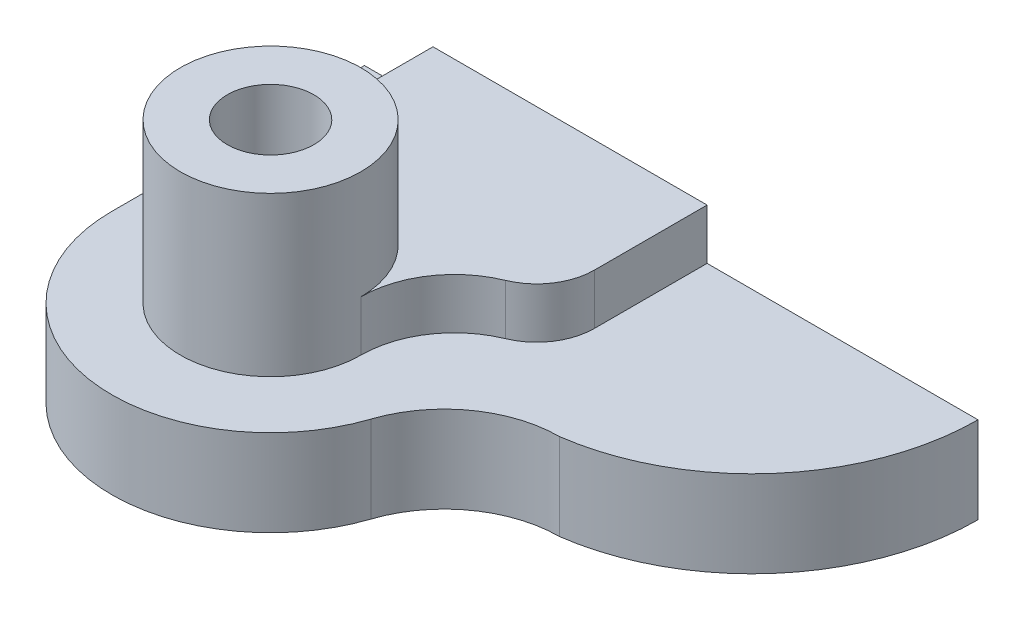
ISO-10303-21;
HEADER;
FILE_DESCRIPTION(('STEP AP214'),'2;1');
FILE_NAME('part.step','',(''),(''),'','','');
FILE_SCHEMA(('AUTOMOTIVE_DESIGN { 1 0 10303 214 1 1 1 1 }'));
ENDSEC;
DATA;
#1=APPLICATION_CONTEXT('core data for automotive mechanical design processes');
#2=APPLICATION_PROTOCOL_DEFINITION('international standard','automotive_design',2000,#1);
#3=PRODUCT_CONTEXT('',#1,'mechanical');
#4=PRODUCT('Part','Part','',(#3));
#5=PRODUCT_RELATED_PRODUCT_CATEGORY('part','',(#4));
#6=PRODUCT_DEFINITION_FORMATION('','',#4);
#7=PRODUCT_DEFINITION_CONTEXT('part definition',#1,'design');
#8=PRODUCT_DEFINITION('design','',#6,#7);
#9=PRODUCT_DEFINITION_SHAPE('','',#8);
#10=(LENGTH_UNIT() NAMED_UNIT(*) SI_UNIT(.MILLI.,.METRE.));
#11=(NAMED_UNIT(*) PLANE_ANGLE_UNIT() SI_UNIT($,.RADIAN.));
#12=(NAMED_UNIT(*) SI_UNIT($,.STERADIAN.) SOLID_ANGLE_UNIT());
#13=UNCERTAINTY_MEASURE_WITH_UNIT(LENGTH_MEASURE(1.E-05),#10,'distance_accuracy_value','');
#14=(GEOMETRIC_REPRESENTATION_CONTEXT(3) GLOBAL_UNCERTAINTY_ASSIGNED_CONTEXT((#13)) GLOBAL_UNIT_ASSIGNED_CONTEXT((#10,
#11,#12)) REPRESENTATION_CONTEXT('',''));
#15=CARTESIAN_POINT('',(0.,0.,0.));
#16=DIRECTION('',(0.,0.,1.));
#17=DIRECTION('',(1.,0.,0.));
#18=AXIS2_PLACEMENT_3D('',#15,#16,#17);
#19=CARTESIAN_POINT('',(36.0555127546399,12.,12.));
#20=DIRECTION('',(0.,-1.,0.));
#21=DIRECTION('',(0.,0.,-1.));
#22=AXIS2_PLACEMENT_3D('',#19,#20,#21);
#23=CYLINDRICAL_SURFACE('',#22,16.);
#24=CARTESIAN_POINT('',(36.0555127546399,0.,12.));
#25=DIRECTION('',(0.,1.,0.));
#26=DIRECTION('',(0.,0.,1.));
#27=AXIS2_PLACEMENT_3D('',#24,#25,#26);
#28=CIRCLE('',#27,16.);
#29=CARTESIAN_POINT('',(36.0555127546399,0.,-4.));
#30=VERTEX_POINT('',#29);
#31=CARTESIAN_POINT('',(20.8742442263705,0.,6.94736842105262));
#32=VERTEX_POINT('',#31);
#33=EDGE_CURVE('E132',#30,#32,#28,.T.);
#34=ORIENTED_EDGE('',*,*,#33,.F.);
#35=DIRECTION('',(0.,-1.,0.));
#36=VECTOR('',#35,1.);
#37=CARTESIAN_POINT('',(36.0555127546399,12.,-4.));
#38=LINE('',#37,#36);
#39=CARTESIAN_POINT('',(36.0555127546399,12.,-4.));
#40=VERTEX_POINT('',#39);
#41=EDGE_CURVE('E11',#40,#30,#38,.T.);
#42=ORIENTED_EDGE('',*,*,#41,.F.);
#43=CARTESIAN_POINT('',(36.0555127546399,12.,12.));
#44=DIRECTION('',(0.,1.,0.));
#45=DIRECTION('',(0.,0.,1.));
#46=AXIS2_PLACEMENT_3D('',#43,#44,#45);
#47=CIRCLE('',#46,16.);
#48=CARTESIAN_POINT('',(20.8742442263705,12.,6.94736842105262));
#49=VERTEX_POINT('',#48);
#50=EDGE_CURVE('E141',#40,#49,#47,.T.);
#51=ORIENTED_EDGE('',*,*,#50,.T.);
#52=DIRECTION('',(0.,-1.,0.));
#53=VECTOR('',#52,1.);
#54=CARTESIAN_POINT('',(20.8742442263705,12.,6.94736842105262));
#55=LINE('',#54,#53);
#56=EDGE_CURVE('E81',#49,#32,#55,.T.);
#57=ORIENTED_EDGE('',*,*,#56,.T.);
#58=EDGE_LOOP('',(#34,#42,#51,#57));
#59=FACE_BOUND('',#58,.T.);
#60=ADVANCED_FACE('F41',(#59),#23,.F.);
#61=CARTESIAN_POINT('',(31.6947950140361,12.,-35.));
#62=DIRECTION('',(0.,-1.,0.));
#63=DIRECTION('',(0.,0.,-1.));
#64=AXIS2_PLACEMENT_3D('',#61,#62,#63);
#65=CYLINDRICAL_SURFACE('',#64,31.3052049859639);
#66=CARTESIAN_POINT('',(31.6947950140361,0.,-35.));
#67=DIRECTION('',(0.,1.,0.));
#68=DIRECTION('',(0.,0.,1.));
#69=AXIS2_PLACEMENT_3D('',#66,#67,#68);
#70=CIRCLE('',#69,31.3052049859639);
#71=CARTESIAN_POINT('',(63.,0.,-35.));
#72=VERTEX_POINT('',#71);
#73=EDGE_CURVE('E135',#72,#30,#70,.F.);
#74=ORIENTED_EDGE('',*,*,#73,.F.);
#75=DIRECTION('',(0.,-1.,0.));
#76=VECTOR('',#75,1.);
#77=CARTESIAN_POINT('',(63.,12.,-35.));
#78=LINE('',#77,#76);
#79=CARTESIAN_POINT('',(63.,12.,-35.));
#80=VERTEX_POINT('',#79);
#81=EDGE_CURVE('E47',#80,#72,#78,.T.);
#82=ORIENTED_EDGE('',*,*,#81,.F.);
#83=CARTESIAN_POINT('',(31.6947950140361,12.,-35.));
#84=DIRECTION('',(0.,1.,0.));
#85=DIRECTION('',(0.,0.,1.));
#86=AXIS2_PLACEMENT_3D('',#83,#84,#85);
#87=CIRCLE('',#86,31.3052049859639);
#88=EDGE_CURVE('E159',#80,#40,#87,.F.);
#89=ORIENTED_EDGE('',*,*,#88,.T.);
#90=ORIENTED_EDGE('',*,*,#41,.T.);
#91=EDGE_LOOP('',(#74,#82,#89,#90));
#92=FACE_BOUND('',#91,.T.);
#93=ADVANCED_FACE('F153',(#92),#65,.T.);
#94=CARTESIAN_POINT('',(0.,12.,-35.));
#95=DIRECTION('',(0.,0.,-1.));
#96=DIRECTION('',(-1.,0.,0.));
#97=AXIS2_PLACEMENT_3D('',#94,#95,#96);
#98=PLANE('',#97);
#99=DIRECTION('',(1.,0.,0.));
#100=VECTOR('',#99,1.);
#101=CARTESIAN_POINT('',(0.,0.,-35.));
#102=LINE('',#101,#100);
#103=CARTESIAN_POINT('',(-22.,0.,-35.));
#104=VERTEX_POINT('',#103);
#105=EDGE_CURVE('E113',#104,#72,#102,.T.);
#106=ORIENTED_EDGE('',*,*,#105,.F.);
#107=DIRECTION('',(0.,-1.,0.));
#108=VECTOR('',#107,1.);
#109=CARTESIAN_POINT('',(-22.,12.,-35.));
#110=LINE('',#109,#108);
#111=CARTESIAN_POINT('',(-22.,12.,-35.));
#112=VERTEX_POINT('',#111);
#113=EDGE_CURVE('E107',#112,#104,#110,.T.);
#114=ORIENTED_EDGE('',*,*,#113,.F.);
#115=DIRECTION('',(1.,0.,0.));
#116=VECTOR('',#115,1.);
#117=CARTESIAN_POINT('',(0.,12.,-35.));
#118=LINE('',#117,#116);
#119=CARTESIAN_POINT('',(-12.5,12.,-35.));
#120=VERTEX_POINT('',#119);
#121=EDGE_CURVE('E114',#112,#120,#118,.T.);
#122=ORIENTED_EDGE('',*,*,#121,.T.);
#123=DIRECTION('',(0.,-1.,0.));
#124=VECTOR('',#123,1.);
#125=CARTESIAN_POINT('',(-12.5,19.,-35.));
#126=LINE('',#125,#124);
#127=CARTESIAN_POINT('',(-12.5,19.,-35.));
#128=VERTEX_POINT('',#127);
#129=EDGE_CURVE('E220',#128,#120,#126,.T.);
#130=ORIENTED_EDGE('',*,*,#129,.F.);
#131=DIRECTION('',(1.,0.,0.));
#132=VECTOR('',#131,1.);
#133=CARTESIAN_POINT('',(0.,19.,-35.));
#134=LINE('',#133,#132);
#135=CARTESIAN_POINT('',(25.4725075103815,19.,-35.));
#136=VERTEX_POINT('',#135);
#137=EDGE_CURVE('E212',#128,#136,#134,.T.);
#138=ORIENTED_EDGE('',*,*,#137,.T.);
#139=DIRECTION('',(0.,-1.,0.));
#140=VECTOR('',#139,1.);
#141=CARTESIAN_POINT('',(25.4725075103815,19.,-35.));
#142=LINE('',#141,#140);
#143=CARTESIAN_POINT('',(25.4725075103815,12.,-35.));
#144=VERTEX_POINT('',#143);
#145=EDGE_CURVE('E221',#136,#144,#142,.T.);
#146=ORIENTED_EDGE('',*,*,#145,.T.);
#147=DIRECTION('',(1.,0.,0.));
#148=VECTOR('',#147,1.);
#149=CARTESIAN_POINT('',(0.,12.,-35.));
#150=LINE('',#149,#148);
#151=EDGE_CURVE('E149',#144,#80,#150,.T.);
#152=ORIENTED_EDGE('',*,*,#151,.T.);
#153=ORIENTED_EDGE('',*,*,#81,.T.);
#154=EDGE_LOOP('',(#106,#114,#122,#130,#138,#146,#152,#153));
#155=FACE_BOUND('',#154,.T.);
#156=ADVANCED_FACE('F109',(#155),#98,.T.);
#157=CARTESIAN_POINT('',(-22.,12.,0.));
#158=DIRECTION('',(1.,0.,0.));
#159=DIRECTION('',(0.,0.,-1.));
#160=AXIS2_PLACEMENT_3D('',#157,#158,#159);
#161=PLANE('',#160);
#162=DIRECTION('',(0.,0.,1.));
#163=VECTOR('',#162,1.);
#164=CARTESIAN_POINT('',(-22.,0.,0.));
#165=LINE('',#164,#163);
#166=CARTESIAN_POINT('',(-22.,0.,0.));
#167=VERTEX_POINT('',#166);
#168=EDGE_CURVE('E76',#104,#167,#165,.T.);
#169=ORIENTED_EDGE('',*,*,#168,.T.);
#170=DIRECTION('',(0.,-1.,0.));
#171=VECTOR('',#170,1.);
#172=CARTESIAN_POINT('',(-22.,12.,0.));
#173=LINE('',#172,#171);
#174=CARTESIAN_POINT('',(-22.,12.,0.));
#175=VERTEX_POINT('',#174);
#176=EDGE_CURVE('E116',#175,#167,#173,.T.);
#177=ORIENTED_EDGE('',*,*,#176,.F.);
#178=DIRECTION('',(0.,0.,1.));
#179=VECTOR('',#178,1.);
#180=CARTESIAN_POINT('',(-22.,12.,0.));
#181=LINE('',#180,#179);
#182=EDGE_CURVE('E119',#112,#175,#181,.T.);
#183=ORIENTED_EDGE('',*,*,#182,.F.);
#184=ORIENTED_EDGE('',*,*,#113,.T.);
#185=EDGE_LOOP('',(#169,#177,#183,#184));
#186=FACE_BOUND('',#185,.T.);
#187=ADVANCED_FACE('F118',(#186),#161,.F.);
#188=CARTESIAN_POINT('',(0.,12.,0.));
#189=DIRECTION('',(0.,-1.,0.));
#190=DIRECTION('',(0.,0.,-1.));
#191=AXIS2_PLACEMENT_3D('',#188,#189,#190);
#192=CYLINDRICAL_SURFACE('',#191,22.);
#193=CARTESIAN_POINT('',(0.,0.,0.));
#194=DIRECTION('',(0.,1.,0.));
#195=DIRECTION('',(0.,0.,1.));
#196=AXIS2_PLACEMENT_3D('',#193,#194,#195);
#197=CIRCLE('',#196,22.);
#198=EDGE_CURVE('E143',#167,#32,#197,.T.);
#199=ORIENTED_EDGE('',*,*,#198,.T.);
#200=ORIENTED_EDGE('',*,*,#56,.F.);
#201=CARTESIAN_POINT('',(0.,12.,0.));
#202=DIRECTION('',(0.,1.,0.));
#203=DIRECTION('',(0.,0.,1.));
#204=AXIS2_PLACEMENT_3D('',#201,#202,#203);
#205=CIRCLE('',#204,22.);
#206=EDGE_CURVE('E60',#175,#49,#205,.T.);
#207=ORIENTED_EDGE('',*,*,#206,.F.);
#208=ORIENTED_EDGE('',*,*,#176,.T.);
#209=EDGE_LOOP('',(#199,#200,#207,#208));
#210=FACE_BOUND('',#209,.T.);
#211=ADVANCED_FACE('F157',(#210),#192,.T.);
#212=CARTESIAN_POINT('',(0.,12.,0.));
#213=DIRECTION('',(0.,1.,0.));
#214=DIRECTION('',(0.,0.,1.));
#215=AXIS2_PLACEMENT_3D('',#212,#213,#214);
#216=PLANE('',#215);
#217=ORIENTED_EDGE('',*,*,#50,.F.);
#218=ORIENTED_EDGE('',*,*,#88,.F.);
#219=ORIENTED_EDGE('',*,*,#151,.F.);
#220=DIRECTION('',(0.,0.,-1.));
#221=VECTOR('',#220,1.);
#222=CARTESIAN_POINT('',(25.4725075103815,12.,0.));
#223=LINE('',#222,#221);
#224=CARTESIAN_POINT('',(25.4725075103815,12.,-19.3867498893706));
#225=VERTEX_POINT('',#224);
#226=EDGE_CURVE('E170',#225,#144,#223,.T.);
#227=ORIENTED_EDGE('',*,*,#226,.F.);
#228=CARTESIAN_POINT('',(17.4725075103815,12.,-19.3867498893706));
#229=DIRECTION('',(0.,1.,0.));
#230=DIRECTION('',(0.,0.,1.));
#231=AXIS2_PLACEMENT_3D('',#228,#229,#230);
#232=CIRCLE('',#231,8.);
#233=CARTESIAN_POINT('',(20.5241216279743,12.,-11.9916399322902));
#234=VERTEX_POINT('',#233);
#235=EDGE_CURVE('E168',#234,#225,#232,.T.);
#236=ORIENTED_EDGE('',*,*,#235,.F.);
#237=CARTESIAN_POINT('',(25.4725075103815,12.,0.));
#238=DIRECTION('',(0.,1.,0.));
#239=DIRECTION('',(0.,0.,1.));
#240=AXIS2_PLACEMENT_3D('',#237,#238,#239);
#241=CIRCLE('',#240,12.9725075103815);
#242=CARTESIAN_POINT('',(12.5,12.,0.));
#243=VERTEX_POINT('',#242);
#244=EDGE_CURVE('E174',#234,#243,#241,.T.);
#245=ORIENTED_EDGE('',*,*,#244,.T.);
#246=CARTESIAN_POINT('',(0.,12.,0.));
#247=DIRECTION('',(0.,1.,0.));
#248=DIRECTION('',(0.,0.,1.));
#249=AXIS2_PLACEMENT_3D('',#246,#247,#248);
#250=CIRCLE('',#249,12.5);
#251=CARTESIAN_POINT('',(-12.5,12.,0.));
#252=VERTEX_POINT('',#251);
#253=EDGE_CURVE('E130',#252,#243,#250,.T.);
#254=ORIENTED_EDGE('',*,*,#253,.F.);
#255=DIRECTION('',(0.,0.,-1.));
#256=VECTOR('',#255,1.);
#257=CARTESIAN_POINT('',(-12.5,12.,0.));
#258=LINE('',#257,#256);
#259=EDGE_CURVE('E124',#252,#120,#258,.T.);
#260=ORIENTED_EDGE('',*,*,#259,.T.);
#261=ORIENTED_EDGE('',*,*,#121,.F.);
#262=ORIENTED_EDGE('',*,*,#182,.T.);
#263=ORIENTED_EDGE('',*,*,#206,.T.);
#264=EDGE_LOOP('',(#217,#218,#219,#227,#236,#245,#254,#260,#261,#262,#263));
#265=FACE_BOUND('',#264,.T.);
#266=ADVANCED_FACE('F125',(#265),#216,.T.);
#267=CARTESIAN_POINT('',(0.,0.,0.));
#268=DIRECTION('',(0.,1.,0.));
#269=DIRECTION('',(0.,0.,1.));
#270=AXIS2_PLACEMENT_3D('',#267,#268,#269);
#271=PLANE('',#270);
#272=ORIENTED_EDGE('',*,*,#105,.T.);
#273=ORIENTED_EDGE('',*,*,#73,.T.);
#274=ORIENTED_EDGE('',*,*,#33,.T.);
#275=ORIENTED_EDGE('',*,*,#198,.F.);
#276=ORIENTED_EDGE('',*,*,#168,.F.);
#277=EDGE_LOOP('',(#272,#273,#274,#275,#276));
#278=FACE_BOUND('',#277,.T.);
#279=CARTESIAN_POINT('',(0.,0.,0.));
#280=DIRECTION('',(0.,1.,0.));
#281=DIRECTION('',(0.,0.,1.));
#282=AXIS2_PLACEMENT_3D('',#279,#280,#281);
#283=CIRCLE('',#282,6.);
#284=CARTESIAN_POINT('',(0.,0.,6.));
#285=VERTEX_POINT('',#284);
#286=EDGE_CURVE('E415',#285,#285,#283,.T.);
#287=ORIENTED_EDGE('',*,*,#286,.T.);
#288=EDGE_LOOP('',(#287));
#289=FACE_BOUND('',#288,.T.);
#290=ADVANCED_FACE('F154',(#278,#289),#271,.F.);
#291=CARTESIAN_POINT('',(25.4725075103815,19.,0.));
#292=DIRECTION('',(0.,-1.,0.));
#293=DIRECTION('',(0.,0.,-1.));
#294=AXIS2_PLACEMENT_3D('',#291,#292,#293);
#295=CYLINDRICAL_SURFACE('',#294,12.9725075103815);
#296=DIRECTION('',(0.,-1.,0.));
#297=VECTOR('',#296,1.);
#298=CARTESIAN_POINT('',(12.5,19.,0.));
#299=LINE('',#298,#297);
#300=CARTESIAN_POINT('',(12.5,19.,0.));
#301=VERTEX_POINT('',#300);
#302=EDGE_CURVE('E181',#301,#243,#299,.T.);
#303=ORIENTED_EDGE('',*,*,#302,.T.);
#304=ORIENTED_EDGE('',*,*,#244,.F.);
#305=DIRECTION('',(0.,-1.,0.));
#306=VECTOR('',#305,1.);
#307=CARTESIAN_POINT('',(20.5241216279743,19.,-11.9916399322902));
#308=LINE('',#307,#306);
#309=CARTESIAN_POINT('',(20.5241216279743,19.,-11.9916399322902));
#310=VERTEX_POINT('',#309);
#311=EDGE_CURVE('E138',#310,#234,#308,.T.);
#312=ORIENTED_EDGE('',*,*,#311,.F.);
#313=CARTESIAN_POINT('',(25.4725075103815,19.,0.));
#314=DIRECTION('',(0.,1.,0.));
#315=DIRECTION('',(0.,0.,1.));
#316=AXIS2_PLACEMENT_3D('',#313,#314,#315);
#317=CIRCLE('',#316,12.9725075103815);
#318=EDGE_CURVE('E240',#310,#301,#317,.T.);
#319=ORIENTED_EDGE('',*,*,#318,.T.);
#320=EDGE_LOOP('',(#303,#304,#312,#319));
#321=FACE_BOUND('',#320,.T.);
#322=ADVANCED_FACE('F237',(#321),#295,.F.);
#323=CARTESIAN_POINT('',(17.4725075103815,19.,-19.3867498893706));
#324=DIRECTION('',(0.,-1.,0.));
#325=DIRECTION('',(0.,0.,-1.));
#326=AXIS2_PLACEMENT_3D('',#323,#324,#325);
#327=CYLINDRICAL_SURFACE('',#326,8.);
#328=ORIENTED_EDGE('',*,*,#235,.T.);
#329=DIRECTION('',(0.,-1.,0.));
#330=VECTOR('',#329,1.);
#331=CARTESIAN_POINT('',(25.4725075103815,19.,-19.3867498893706));
#332=LINE('',#331,#330);
#333=CARTESIAN_POINT('',(25.4725075103815,19.,-19.3867498893706));
#334=VERTEX_POINT('',#333);
#335=EDGE_CURVE('E223',#334,#225,#332,.T.);
#336=ORIENTED_EDGE('',*,*,#335,.F.);
#337=CARTESIAN_POINT('',(17.4725075103815,19.,-19.3867498893706));
#338=DIRECTION('',(0.,1.,0.));
#339=DIRECTION('',(0.,0.,1.));
#340=AXIS2_PLACEMENT_3D('',#337,#338,#339);
#341=CIRCLE('',#340,8.);
#342=EDGE_CURVE('E232',#310,#334,#341,.T.);
#343=ORIENTED_EDGE('',*,*,#342,.F.);
#344=ORIENTED_EDGE('',*,*,#311,.T.);
#345=EDGE_LOOP('',(#328,#336,#343,#344));
#346=FACE_BOUND('',#345,.T.);
#347=ADVANCED_FACE('F231',(#346),#327,.T.);
#348=CARTESIAN_POINT('',(25.4725075103815,19.,0.));
#349=DIRECTION('',(-1.,0.,0.));
#350=DIRECTION('',(0.,0.,1.));
#351=AXIS2_PLACEMENT_3D('',#348,#349,#350);
#352=PLANE('',#351);
#353=ORIENTED_EDGE('',*,*,#226,.T.);
#354=ORIENTED_EDGE('',*,*,#145,.F.);
#355=DIRECTION('',(0.,0.,-1.));
#356=VECTOR('',#355,1.);
#357=CARTESIAN_POINT('',(25.4725075103815,19.,0.));
#358=LINE('',#357,#356);
#359=EDGE_CURVE('E238',#334,#136,#358,.T.);
#360=ORIENTED_EDGE('',*,*,#359,.F.);
#361=ORIENTED_EDGE('',*,*,#335,.T.);
#362=EDGE_LOOP('',(#353,#354,#360,#361));
#363=FACE_BOUND('',#362,.T.);
#364=ADVANCED_FACE('F246',(#363),#352,.F.);
#365=CARTESIAN_POINT('',(-12.5,19.,0.));
#366=DIRECTION('',(-1.,0.,0.));
#367=DIRECTION('',(0.,0.,1.));
#368=AXIS2_PLACEMENT_3D('',#365,#366,#367);
#369=PLANE('',#368);
#370=ORIENTED_EDGE('',*,*,#129,.T.);
#371=ORIENTED_EDGE('',*,*,#259,.F.);
#372=DIRECTION('',(0.,-1.,0.));
#373=VECTOR('',#372,1.);
#374=CARTESIAN_POINT('',(-12.5,19.,0.));
#375=LINE('',#374,#373);
#376=CARTESIAN_POINT('',(-12.5,19.,0.));
#377=VERTEX_POINT('',#376);
#378=EDGE_CURVE('E186',#377,#252,#375,.T.);
#379=ORIENTED_EDGE('',*,*,#378,.F.);
#380=DIRECTION('',(0.,0.,-1.));
#381=VECTOR('',#380,1.);
#382=CARTESIAN_POINT('',(-12.5,19.,0.));
#383=LINE('',#382,#381);
#384=EDGE_CURVE('E207',#377,#128,#383,.T.);
#385=ORIENTED_EDGE('',*,*,#384,.T.);
#386=EDGE_LOOP('',(#370,#371,#379,#385));
#387=FACE_BOUND('',#386,.T.);
#388=ADVANCED_FACE('F216',(#387),#369,.T.);
#389=CARTESIAN_POINT('',(0.,19.,0.));
#390=DIRECTION('',(0.,1.,0.));
#391=DIRECTION('',(0.,0.,1.));
#392=AXIS2_PLACEMENT_3D('',#389,#390,#391);
#393=PLANE('',#392);
#394=ORIENTED_EDGE('',*,*,#318,.F.);
#395=ORIENTED_EDGE('',*,*,#342,.T.);
#396=ORIENTED_EDGE('',*,*,#359,.T.);
#397=ORIENTED_EDGE('',*,*,#137,.F.);
#398=ORIENTED_EDGE('',*,*,#384,.F.);
#399=CARTESIAN_POINT('',(0.,19.,0.));
#400=DIRECTION('',(0.,1.,0.));
#401=DIRECTION('',(0.,0.,1.));
#402=AXIS2_PLACEMENT_3D('',#399,#400,#401);
#403=CIRCLE('',#402,12.5);
#404=EDGE_CURVE('E215',#301,#377,#403,.T.);
#405=ORIENTED_EDGE('',*,*,#404,.F.);
#406=EDGE_LOOP('',(#394,#395,#396,#397,#398,#405));
#407=FACE_BOUND('',#406,.T.);
#408=ADVANCED_FACE('F211',(#407),#393,.T.);
#409=CARTESIAN_POINT('',(0.,34.,0.));
#410=DIRECTION('',(0.,1.,0.));
#411=DIRECTION('',(0.,0.,1.));
#412=AXIS2_PLACEMENT_3D('',#409,#410,#411);
#413=PLANE('',#412);
#414=CARTESIAN_POINT('',(0.,34.,0.));
#415=DIRECTION('',(0.,1.,0.));
#416=DIRECTION('',(0.,0.,1.));
#417=AXIS2_PLACEMENT_3D('',#414,#415,#416);
#418=CIRCLE('',#417,12.5);
#419=CARTESIAN_POINT('',(0.,34.,12.5));
#420=VERTEX_POINT('',#419);
#421=EDGE_CURVE('E236',#420,#420,#418,.T.);
#422=ORIENTED_EDGE('',*,*,#421,.T.);
#423=EDGE_LOOP('',(#422));
#424=FACE_BOUND('',#423,.T.);
#425=CARTESIAN_POINT('',(0.,34.,0.));
#426=DIRECTION('',(0.,1.,0.));
#427=DIRECTION('',(0.,0.,1.));
#428=AXIS2_PLACEMENT_3D('',#425,#426,#427);
#429=CIRCLE('',#428,6.);
#430=CARTESIAN_POINT('',(0.,34.,6.));
#431=VERTEX_POINT('',#430);
#432=EDGE_CURVE('E244',#431,#431,#429,.T.);
#433=ORIENTED_EDGE('',*,*,#432,.F.);
#434=EDGE_LOOP('',(#433));
#435=FACE_BOUND('',#434,.T.);
#436=ADVANCED_FACE('F291',(#424,#435),#413,.T.);
#437=CARTESIAN_POINT('',(0.,34.,0.));
#438=DIRECTION('',(0.,-1.,0.));
#439=DIRECTION('',(0.,0.,-1.));
#440=AXIS2_PLACEMENT_3D('',#437,#438,#439);
#441=CYLINDRICAL_SURFACE('',#440,12.5);
#442=ORIENTED_EDGE('',*,*,#302,.F.);
#443=ORIENTED_EDGE('',*,*,#404,.T.);
#444=ORIENTED_EDGE('',*,*,#378,.T.);
#445=ORIENTED_EDGE('',*,*,#253,.T.);
#446=EDGE_LOOP('',(#442,#443,#444,#445));
#447=FACE_BOUND('',#446,.T.);
#448=ORIENTED_EDGE('',*,*,#421,.F.);
#449=EDGE_LOOP('',(#448));
#450=FACE_BOUND('',#449,.T.);
#451=ADVANCED_FACE('F176',(#447,#450),#441,.T.);
#452=CARTESIAN_POINT('',(0.,34.,0.));
#453=DIRECTION('',(0.,-1.,0.));
#454=DIRECTION('',(0.,0.,-1.));
#455=AXIS2_PLACEMENT_3D('',#452,#453,#454);
#456=CYLINDRICAL_SURFACE('',#455,6.);
#457=ORIENTED_EDGE('',*,*,#432,.T.);
#458=EDGE_LOOP('',(#457));
#459=FACE_BOUND('',#458,.T.);
#460=ORIENTED_EDGE('',*,*,#286,.F.);
#461=EDGE_LOOP('',(#460));
#462=FACE_BOUND('',#461,.T.);
#463=ADVANCED_FACE('F306',(#459,#462),#456,.F.);
#464=CLOSED_SHELL('',(#60,#93,#156,#187,#211,#266,#290,#322,#347,#364,#388,#408,#436,#451,#463));
#465=MANIFOLD_SOLID_BREP('B2',#464);
#466=ADVANCED_BREP_SHAPE_REPRESENTATION('',(#18,#465),#14);
#467=SHAPE_DEFINITION_REPRESENTATION(#9,#466);
ENDSEC;
END-ISO-10303-21;
